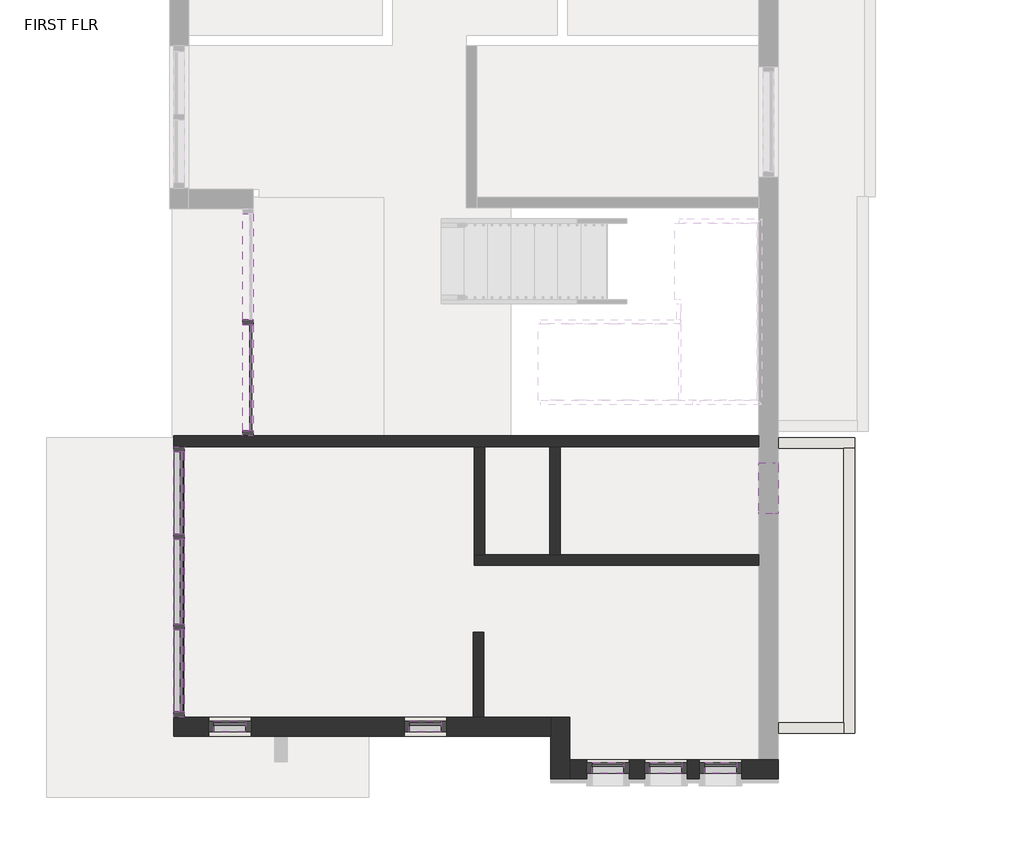
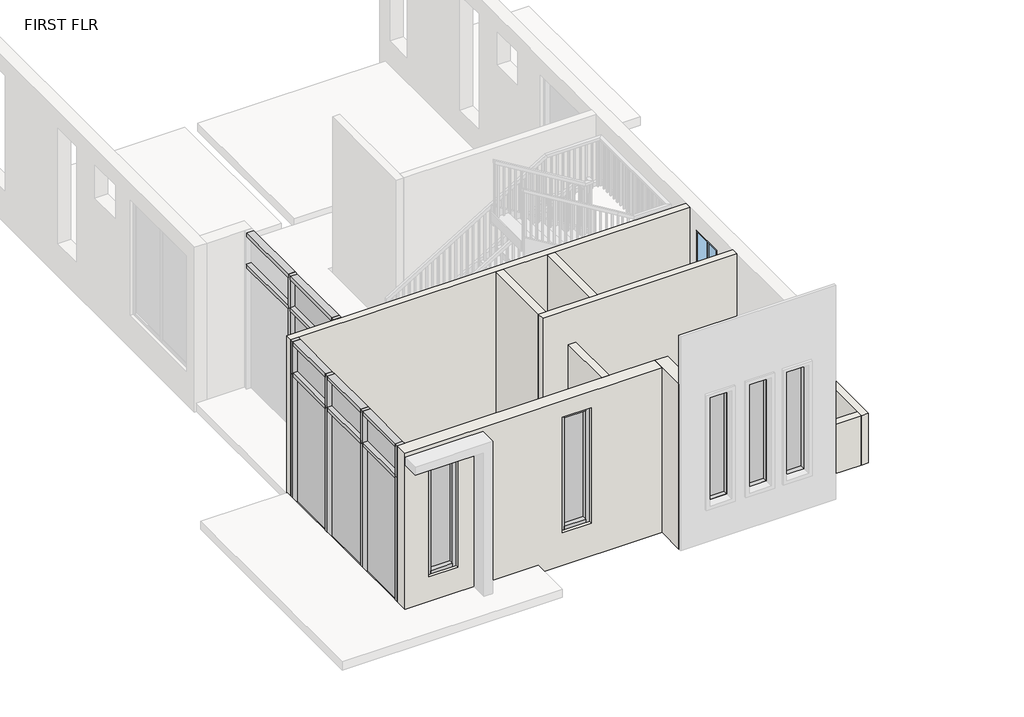
# One storey, part 1 of 4: 46 members, 13 plates, 11 walls, 1 window.
"""IFC4 building model written with IfcOpenShell, lengths in millimetres."""

from ifc_helpers import new_model, si_unit, frame, origin, place, context, project, spatial, polyline, outline, extrude, faceted_brep, transform, mapped, element, save
from components import member_f0fea5a5, member_ee409385, member_2af3cda3, member_40129ecf, member_6e77e263, member_47bfaf8a, member_1093a910, member_585633ab, member_389f1ce1, member_852ada5c, member_dfe75557, member_3374d9b6, system_panel_glazed_2be43394, system_panel_glazed_82b35773, system_panel_glazed_8cf484b6, system_panel_glazed_73690fa1, system_panel_glazed_b4437c67, system_panel_glazed_c5c5478c, system_panel_glazed_dc74cd20, window_80340324

model = new_model("IFC4")

# Units and contexts
model_context = context("Model", 3, world=origin())
ifc_project = project(units=[si_unit("LENGTHUNIT", "METRE", prefix="MILLI")], contexts=[model_context])

# Site, building, storey
site = spatial("IfcSite", under=ifc_project)
building = spatial("IfcBuilding", under=site)
storey = spatial("IfcBuildingStorey", under=building, Name="FIRST FLR", Elevation=3048.0)

# Members
placement = place(None, origin())
member_shape = member_f0fea5a5(model_context)
element("IfcMember", 1, ObjectType="Rectangular Mullion : 2.5\" x 5\" rectangular", at=placement, inside=storey, context=model_context, shape_type="MappedRepresentation", body=[
    mapped(member_shape, transform((-12015.640556, -6619.6163702, 3048.0), x_axis=(0.0, -1.0, 0.0), y_axis=(-1.0, 0.0, 0.0), z_axis=(0.0, 0.0, -1.0))),
])
element("IfcMember", 2, ObjectType="Rectangular Mullion : 2.5\" x 5\" rectangular", at=placement, inside=storey, context=model_context, shape_type="MappedRepresentation", body=[
    mapped(member_shape, transform((-12844.3906521, -9183.83582, 3048.0), x_axis=(0.0, -1.0, 0.0), y_axis=(-1.0, 0.0, 0.0), z_axis=(0.0, 0.0, -1.0))),
])
element("IfcMember", 3, ObjectType="Rectangular Mullion : 2.5\" x 5\" rectangular", at=placement, inside=storey, context=model_context, shape_type="MappedRepresentation", body=[
    mapped(member_shape, transform((-12844.3906521, -10261.7405605, 3048.0), x_axis=(0.0, -1.0, 0.0), y_axis=(-1.0, 0.0, 0.0), z_axis=(0.0, 0.0, -1.0))),
])
member_2_shape = member_ee409385(model_context)
element("IfcMember", 4, ObjectType="Rectangular Mullion : 2.5\" x 5\" rectangular", at=placement, inside=storey, context=model_context, shape_type="MappedRepresentation", body=[
    mapped(member_2_shape, transform((-12015.640556, -7978.9310793, 3048.0), x_axis=(0.0, -1.0, 0.0), y_axis=(-1.0, 0.0, 0.0), z_axis=(0.0, 0.0, -1.0))),
])
element("IfcMember", 5, ObjectType="Rectangular Mullion : 2.5\" x 5\" rectangular", at=placement, inside=storey, context=model_context, shape_type="MappedRepresentation", body=[
    mapped(member_2_shape, transform((-12844.3906521, -11339.6453012, 3048.0), x_axis=(0.0, -1.0, 0.0), y_axis=(-1.0, 0.0, 0.0), z_axis=(0.0, 0.0, -1.0))),
])
element("IfcMember", 6, ObjectType="Rectangular Mullion : 2.5\" x 5\" rectangular", at=placement, inside=storey, context=model_context, shape_type="MappedRepresentation", body=[
    mapped(member_2_shape, transform((-12844.3906521, -8105.9310793, 5486.4), x_axis=(0.0, 1.0, 0.0), y_axis=(-1.0, 0.0, 0.0), z_axis=(0.0, 0.0, 1.0))),
])
member_3_shape = member_2af3cda3(model_context)
element("IfcMember", 7, ObjectType="Rectangular Mullion : 2.5\" x 5\" rectangular", at=placement, inside=storey, context=model_context, shape_type="MappedRepresentation", body=[
    mapped(member_3_shape, transform((-12015.640556, -7915.4310793, 6096.0), x_axis=(0.0, 0.0, 1.0), y_axis=(-1.0, 0.0, 0.0), z_axis=(0.0, -1.0, 0.0))),
])
element("IfcMember", 8, ObjectType="Rectangular Mullion : 2.5\" x 5\" rectangular", at=placement, inside=storey, context=model_context, shape_type="MappedRepresentation", body=[
    mapped(member_3_shape, transform((-12015.640556, -6587.8663702, 6096.0), x_axis=(0.0, 0.0, 1.0), y_axis=(-1.0, 0.0, 0.0), z_axis=(0.0, -1.0, 0.0))),
])
element("IfcMember", 9, ObjectType="Rectangular Mullion : 2.5\" x 5\" rectangular", at=placement, inside=storey, context=model_context, shape_type="MappedRepresentation", body=[
    mapped(member_3_shape, transform((-12015.640556, -6651.3663702, 3048.0), x_axis=(0.0, 0.0, -1.0), y_axis=(-1.0, 0.0, 0.0), z_axis=(0.0, 1.0, 0.0))),
])
member_4_shape = member_40129ecf(model_context)
element("IfcMember", 10, ObjectType="Rectangular Mullion : 2.5\" x 5\" rectangular", at=placement, inside=storey, context=model_context, shape_type="MappedRepresentation", body=[
    mapped(member_4_shape, transform((-12015.640556, -6587.8663702, 5486.4), x_axis=(0.0, 0.0, 1.0), y_axis=(-1.0, 0.0, 0.0), z_axis=(0.0, -1.0, 0.0))),
])
element("IfcMember", 11, ObjectType="Rectangular Mullion : 2.5\" x 5\" rectangular", at=placement, inside=storey, context=model_context, shape_type="MappedRepresentation", body=[
    mapped(member_4_shape, transform((-12015.640556, -7915.4310793, 5486.4), x_axis=(0.0, 0.0, 1.0), y_axis=(-1.0, 0.0, 0.0), z_axis=(0.0, -1.0, 0.0))),
])
member_5_shape = member_6e77e263(model_context)
element("IfcMember", 12, ObjectType="Rectangular Mullion : 2.5\" x 5\" rectangular", at=placement, inside=storey, context=model_context, shape_type="MappedRepresentation", body=[
    mapped(member_5_shape, transform((-12015.640556, -6619.6163702, 5486.4), x_axis=(0.0, -1.0, 0.0), y_axis=(-1.0, 0.0, 0.0), z_axis=(0.0, 0.0, -1.0))),
])
element("IfcMember", 13, ObjectType="Rectangular Mullion : 2.5\" x 5\" rectangular", at=placement, inside=storey, context=model_context, shape_type="MappedRepresentation", body=[
    mapped(member_5_shape, transform((-12844.3906521, -9183.83582, 5486.4), x_axis=(0.0, -1.0, 0.0), y_axis=(-1.0, 0.0, 0.0), z_axis=(0.0, 0.0, -1.0))),
])
element("IfcMember", 14, ObjectType="Rectangular Mullion : 2.5\" x 5\" rectangular", at=placement, inside=storey, context=model_context, shape_type="MappedRepresentation", body=[
    mapped(member_5_shape, transform((-12844.3906521, -10261.7405605, 5486.4), x_axis=(0.0, -1.0, 0.0), y_axis=(-1.0, 0.0, 0.0), z_axis=(0.0, 0.0, -1.0))),
])
member_6_shape = member_47bfaf8a(model_context)
element("IfcMember", 15, ObjectType="Rectangular Mullion : 2.5\" x 5\" rectangular", at=placement, inside=storey, context=model_context, shape_type="MappedRepresentation", body=[
    mapped(member_6_shape, transform((-12844.3906521, -8105.9310793, 6096.0), x_axis=(0.0, 1.0, 0.0), y_axis=(-1.0, 0.0, 0.0), z_axis=(0.0, 0.0, 1.0))),
])
element("IfcMember", 16, ObjectType="Rectangular Mullion : 2.5\" x 5\" rectangular", at=placement, inside=storey, context=model_context, shape_type="MappedRepresentation", body=[
    mapped(member_6_shape, transform((-12015.640556, -7978.9310793, 5486.4), x_axis=(0.0, -1.0, 0.0), y_axis=(-1.0, 0.0, 0.0), z_axis=(0.0, 0.0, -1.0))),
])
element("IfcMember", 17, ObjectType="Rectangular Mullion : 2.5\" x 5\" rectangular", at=placement, inside=storey, context=model_context, shape_type="MappedRepresentation", body=[
    mapped(member_6_shape, transform((-12844.3906521, -11339.6453012, 5486.4), x_axis=(0.0, -1.0, 0.0), y_axis=(-1.0, 0.0, 0.0), z_axis=(0.0, 0.0, -1.0))),
])
member_7_shape = member_1093a910(model_context)
element("IfcMember", 18, ObjectType="Rectangular Mullion : 2.5\" x 5\" rectangular", at=placement, inside=storey, context=model_context, shape_type="MappedRepresentation", body=[
    mapped(member_7_shape, transform((-12844.3906521, -11276.1453012, 6096.0), x_axis=(0.0, 0.0, 1.0), y_axis=(-1.0, 0.0, 0.0), z_axis=(0.0, -1.0, 0.0))),
])
element("IfcMember", 19, ObjectType="Rectangular Mullion : 2.5\" x 5\" rectangular", at=placement, inside=storey, context=model_context, shape_type="MappedRepresentation", body=[
    mapped(member_7_shape, transform((-12844.3906521, -9152.08582, 6096.0), x_axis=(0.0, 0.0, 1.0), y_axis=(-1.0, 0.0, 0.0), z_axis=(0.0, -1.0, 0.0))),
])
element("IfcMember", 20, ObjectType="Rectangular Mullion : 2.5\" x 5\" rectangular", at=placement, inside=storey, context=model_context, shape_type="MappedRepresentation", body=[
    mapped(member_7_shape, transform((-12844.3906521, -8169.4310793, 3048.0), x_axis=(0.0, 0.0, -1.0), y_axis=(-1.0, 0.0, 0.0), z_axis=(0.0, 1.0, 0.0))),
])
element("IfcMember", 21, ObjectType="Rectangular Mullion : 2.5\" x 5\" rectangular", at=placement, inside=storey, context=model_context, shape_type="MappedRepresentation", body=[
    mapped(member_7_shape, transform((-12844.3906521, -10293.4905605, 3048.0), x_axis=(0.0, 0.0, -1.0), y_axis=(-1.0, 0.0, 0.0), z_axis=(0.0, 1.0, 0.0))),
])
member_8_shape = member_585633ab(model_context)
element("IfcMember", 22, ObjectType="Rectangular Mullion : 2.5\" x 5\" rectangular", at=placement, inside=storey, context=model_context, shape_type="MappedRepresentation", body=[
    mapped(member_8_shape, transform((-12844.3906521, -10229.9905605, 6096.0), x_axis=(0.0, 0.0, 1.0), y_axis=(-1.0, 0.0, 0.0), z_axis=(0.0, -1.0, 0.0))),
])
element("IfcMember", 23, ObjectType="Rectangular Mullion : 2.5\" x 5\" rectangular", at=placement, inside=storey, context=model_context, shape_type="MappedRepresentation", body=[
    mapped(member_8_shape, transform((-12844.3906521, -9215.58582, 3048.0), x_axis=(0.0, 0.0, -1.0), y_axis=(-1.0, 0.0, 0.0), z_axis=(0.0, 1.0, 0.0))),
])
member_9_shape = member_389f1ce1(model_context)
element("IfcMember", 24, ObjectType="Rectangular Mullion : 2.5\" x 5\" rectangular", at=placement, inside=storey, context=model_context, shape_type="MappedRepresentation", body=[
    mapped(member_9_shape, transform((-12844.3906521, -9152.08582, 5486.4), x_axis=(0.0, 0.0, 1.0), y_axis=(-1.0, 0.0, 0.0), z_axis=(0.0, -1.0, 0.0))),
])
element("IfcMember", 25, ObjectType="Rectangular Mullion : 2.5\" x 5\" rectangular", at=placement, inside=storey, context=model_context, shape_type="MappedRepresentation", body=[
    mapped(member_9_shape, transform((-12844.3906521, -11276.1453012, 5486.4), x_axis=(0.0, 0.0, 1.0), y_axis=(-1.0, 0.0, 0.0), z_axis=(0.0, -1.0, 0.0))),
])
member_10_shape = member_852ada5c(model_context)
element("IfcMember", 26, ObjectType="Rectangular Mullion : 2.5\" x 5\" rectangular", at=placement, inside=storey, context=model_context, shape_type="MappedRepresentation", body=[
    mapped(member_10_shape, transform((-12844.3906521, -10229.9905605, 5486.4), x_axis=(0.0, 0.0, 1.0), y_axis=(-1.0, 0.0, 0.0), z_axis=(0.0, -1.0, 0.0))),
])
member_11_shape = member_dfe75557(model_context)
element("IfcMember", 27, ObjectType="Rectangular Mullion : 2.5\" x 5\" rectangular", at=placement, inside=storey, context=model_context, shape_type="MappedRepresentation", body=[
    mapped(member_11_shape, transform((-7523.7171142, -11945.8509606, 5791.2), x_axis=(0.0, 0.0, 1.0), y_axis=(0.0, -1.0, 0.0), z_axis=(1.0, 0.0, 0.0))),
])
element("IfcMember", 28, ObjectType="Rectangular Mullion : 2.5\" x 5\" rectangular", at=placement, inside=storey, context=model_context, shape_type="MappedRepresentation", body=[
    mapped(member_11_shape, transform((-6831.5671142, -11945.8509606, 5791.2), x_axis=(0.0, 0.0, 1.0), y_axis=(0.0, -1.0, 0.0), z_axis=(1.0, 0.0, 0.0))),
])
element("IfcMember", 29, ObjectType="Rectangular Mullion : 2.5\" x 5\" rectangular", at=placement, inside=storey, context=model_context, shape_type="MappedRepresentation", body=[
    mapped(member_11_shape, transform((-6177.5171142, -11945.8509606, 5791.2), x_axis=(0.0, 0.0, 1.0), y_axis=(0.0, -1.0, 0.0), z_axis=(1.0, 0.0, 0.0))),
])
element("IfcMember", 30, ObjectType="Rectangular Mullion : 2.5\" x 5\" rectangular", at=placement, inside=storey, context=model_context, shape_type="MappedRepresentation", body=[
    mapped(member_11_shape, transform((-9707.4906521, -11453.9453012, 5791.2), x_axis=(0.0, 0.0, 1.0), y_axis=(0.0, -1.0, 0.0), z_axis=(1.0, 0.0, 0.0))),
])
element("IfcMember", 31, ObjectType="Rectangular Mullion : 2.5\" x 5\" rectangular", at=placement, inside=storey, context=model_context, shape_type="MappedRepresentation", body=[
    mapped(member_11_shape, transform((-12044.2906521, -11453.9453012, 5791.2), x_axis=(0.0, 0.0, 1.0), y_axis=(0.0, -1.0, 0.0), z_axis=(1.0, 0.0, 0.0))),
])
element("IfcMember", 32, ObjectType="Rectangular Mullion : 2.5\" x 5\" rectangular", at=placement, inside=storey, context=model_context, shape_type="MappedRepresentation", body=[
    mapped(member_11_shape, transform((-7904.7171142, -11945.8509606, 3657.6), x_axis=(0.0, 0.0, -1.0), y_axis=(0.0, -1.0, 0.0), z_axis=(-1.0, 0.0, 0.0))),
])
element("IfcMember", 33, ObjectType="Rectangular Mullion : 2.5\" x 5\" rectangular", at=placement, inside=storey, context=model_context, shape_type="MappedRepresentation", body=[
    mapped(member_11_shape, transform((-7212.5671142, -11945.8509606, 3657.6), x_axis=(0.0, 0.0, -1.0), y_axis=(0.0, -1.0, 0.0), z_axis=(-1.0, 0.0, 0.0))),
])
element("IfcMember", 34, ObjectType="Rectangular Mullion : 2.5\" x 5\" rectangular", at=placement, inside=storey, context=model_context, shape_type="MappedRepresentation", body=[
    mapped(member_11_shape, transform((-6558.5171142, -11945.8509606, 3657.6), x_axis=(0.0, 0.0, -1.0), y_axis=(0.0, -1.0, 0.0), z_axis=(-1.0, 0.0, 0.0))),
])
element("IfcMember", 35, ObjectType="Rectangular Mullion : 2.5\" x 5\" rectangular", at=placement, inside=storey, context=model_context, shape_type="MappedRepresentation", body=[
    mapped(member_11_shape, transform((-10088.4906521, -11453.9453012, 3657.6), x_axis=(0.0, 0.0, -1.0), y_axis=(0.0, -1.0, 0.0), z_axis=(-1.0, 0.0, 0.0))),
])
element("IfcMember", 36, ObjectType="Rectangular Mullion : 2.5\" x 5\" rectangular", at=placement, inside=storey, context=model_context, shape_type="MappedRepresentation", body=[
    mapped(member_11_shape, transform((-12425.2906521, -11453.9453012, 3657.6), x_axis=(0.0, 0.0, -1.0), y_axis=(0.0, -1.0, 0.0), z_axis=(-1.0, 0.0, 0.0))),
])
member_12_shape = member_3374d9b6(model_context)
element("IfcMember", 37, ObjectType="Rectangular Mullion : 2.5\" x 5\" rectangular", at=placement, inside=storey, context=model_context, shape_type="MappedRepresentation", body=[
    mapped(member_12_shape, transform((-7460.2171142, -11945.8509606, 3657.6), x_axis=(1.0, 0.0, 0.0), y_axis=(0.0, -1.0, 0.0), z_axis=(0.0, 0.0, -1.0))),
])
element("IfcMember", 38, ObjectType="Rectangular Mullion : 2.5\" x 5\" rectangular", at=placement, inside=storey, context=model_context, shape_type="MappedRepresentation", body=[
    mapped(member_12_shape, transform((-6768.0671142, -11945.8509606, 3657.6), x_axis=(1.0, 0.0, 0.0), y_axis=(0.0, -1.0, 0.0), z_axis=(0.0, 0.0, -1.0))),
])
element("IfcMember", 39, ObjectType="Rectangular Mullion : 2.5\" x 5\" rectangular", at=placement, inside=storey, context=model_context, shape_type="MappedRepresentation", body=[
    mapped(member_12_shape, transform((-6114.0171142, -11945.8509606, 3657.6), x_axis=(1.0, 0.0, 0.0), y_axis=(0.0, -1.0, 0.0), z_axis=(0.0, 0.0, -1.0))),
])
element("IfcMember", 40, ObjectType="Rectangular Mullion : 2.5\" x 5\" rectangular", at=placement, inside=storey, context=model_context, shape_type="MappedRepresentation", body=[
    mapped(member_12_shape, transform((-9643.9906521, -11453.9453012, 3657.6), x_axis=(1.0, 0.0, 0.0), y_axis=(0.0, -1.0, 0.0), z_axis=(0.0, 0.0, -1.0))),
])
element("IfcMember", 41, ObjectType="Rectangular Mullion : 2.5\" x 5\" rectangular", at=placement, inside=storey, context=model_context, shape_type="MappedRepresentation", body=[
    mapped(member_12_shape, transform((-11980.7906521, -11453.9453012, 3657.6), x_axis=(1.0, 0.0, 0.0), y_axis=(0.0, -1.0, 0.0), z_axis=(0.0, 0.0, -1.0))),
])
element("IfcMember", 42, ObjectType="Rectangular Mullion : 2.5\" x 5\" rectangular", at=placement, inside=storey, context=model_context, shape_type="MappedRepresentation", body=[
    mapped(member_12_shape, transform((-7968.2171142, -11945.8509606, 5791.2), x_axis=(-1.0, 0.0, 0.0), y_axis=(0.0, -1.0, 0.0), z_axis=(0.0, 0.0, 1.0))),
])
element("IfcMember", 43, ObjectType="Rectangular Mullion : 2.5\" x 5\" rectangular", at=placement, inside=storey, context=model_context, shape_type="MappedRepresentation", body=[
    mapped(member_12_shape, transform((-7276.0671142, -11945.8509606, 5791.2), x_axis=(-1.0, 0.0, 0.0), y_axis=(0.0, -1.0, 0.0), z_axis=(0.0, 0.0, 1.0))),
])
element("IfcMember", 44, ObjectType="Rectangular Mullion : 2.5\" x 5\" rectangular", at=placement, inside=storey, context=model_context, shape_type="MappedRepresentation", body=[
    mapped(member_12_shape, transform((-6622.0171142, -11945.8509606, 5791.2), x_axis=(-1.0, 0.0, 0.0), y_axis=(0.0, -1.0, 0.0), z_axis=(0.0, 0.0, 1.0))),
])
element("IfcMember", 45, ObjectType="Rectangular Mullion : 2.5\" x 5\" rectangular", at=placement, inside=storey, context=model_context, shape_type="MappedRepresentation", body=[
    mapped(member_12_shape, transform((-10151.9906521, -11453.9453012, 5791.2), x_axis=(-1.0, 0.0, 0.0), y_axis=(0.0, -1.0, 0.0), z_axis=(0.0, 0.0, 1.0))),
])
element("IfcMember", 46, ObjectType="Rectangular Mullion : 2.5\" x 5\" rectangular", at=placement, inside=storey, context=model_context, shape_type="MappedRepresentation", body=[
    mapped(member_12_shape, transform((-12488.7906521, -11453.9453012, 5791.2), x_axis=(-1.0, 0.0, 0.0), y_axis=(0.0, -1.0, 0.0), z_axis=(0.0, 0.0, 1.0))),
])

# Plates
system_panel_glazed_shape = system_panel_glazed_2be43394(model_context)
element("IfcPlate", 47, ObjectType="System Panel : Glazed", at=placement, inside=storey, context=model_context, shape_type="MappedRepresentation", body=[
    mapped(system_panel_glazed_shape, transform((-12015.640556, -7283.3987247, 3111.5), x_axis=(0.0, -1.0, 0.0), y_axis=(1.0, 0.0, 0.0), z_axis=(0.0, 0.0, 1.0))),
])
system_panel_glazed_2_shape = system_panel_glazed_82b35773(model_context)
element("IfcPlate", 48, ObjectType="System Panel : Glazed", at=placement, inside=storey, context=model_context, shape_type="MappedRepresentation", body=[
    mapped(system_panel_glazed_2_shape, transform((-12015.640556, -7283.3987247, 5518.15), x_axis=(0.0, -1.0, 0.0), y_axis=(1.0, 0.0, 0.0), z_axis=(0.0, 0.0, 1.0))),
])
system_panel_glazed_3_shape = system_panel_glazed_8cf484b6(model_context)
element("IfcPlate", 49, ObjectType="System Panel : Glazed", at=placement, inside=storey, context=model_context, shape_type="MappedRepresentation", body=[
    mapped(system_panel_glazed_3_shape, transform((-12844.3906521, -8660.7584496, 3111.5), x_axis=(0.0, -1.0, 0.0), y_axis=(1.0, 0.0, 0.0), z_axis=(0.0, 0.0, 1.0))),
])
element("IfcPlate", 50, ObjectType="System Panel : Glazed", at=placement, inside=storey, context=model_context, shape_type="MappedRepresentation", body=[
    mapped(system_panel_glazed_3_shape, transform((-12844.3906521, -10784.8179308, 3111.5), x_axis=(0.0, -1.0, 0.0), y_axis=(1.0, 0.0, 0.0), z_axis=(0.0, 0.0, 1.0))),
])
system_panel_glazed_4_shape = system_panel_glazed_73690fa1(model_context)
element("IfcPlate", 51, ObjectType="System Panel : Glazed", at=placement, inside=storey, context=model_context, shape_type="MappedRepresentation", body=[
    mapped(system_panel_glazed_4_shape, transform((-12844.3906521, -9722.7881902, 3111.5), x_axis=(0.0, -1.0, 0.0), y_axis=(1.0, 0.0, 0.0), z_axis=(0.0, 0.0, 1.0))),
])
system_panel_glazed_5_shape = system_panel_glazed_b4437c67(model_context)
element("IfcPlate", 52, ObjectType="System Panel : Glazed", at=placement, inside=storey, context=model_context, shape_type="MappedRepresentation", body=[
    mapped(system_panel_glazed_5_shape, transform((-12844.3906521, -8660.7584496, 5518.15), x_axis=(0.0, -1.0, 0.0), y_axis=(1.0, 0.0, 0.0), z_axis=(0.0, 0.0, 1.0))),
])
element("IfcPlate", 53, ObjectType="System Panel : Glazed", at=placement, inside=storey, context=model_context, shape_type="MappedRepresentation", body=[
    mapped(system_panel_glazed_5_shape, transform((-12844.3906521, -10784.8179308, 5518.15), x_axis=(0.0, -1.0, 0.0), y_axis=(1.0, 0.0, 0.0), z_axis=(0.0, 0.0, 1.0))),
])
system_panel_glazed_6_shape = system_panel_glazed_c5c5478c(model_context)
element("IfcPlate", 54, ObjectType="System Panel : Glazed", at=placement, inside=storey, context=model_context, shape_type="MappedRepresentation", body=[
    mapped(system_panel_glazed_6_shape, transform((-12844.3906521, -9722.7881902, 5518.15), x_axis=(0.0, -1.0, 0.0), y_axis=(1.0, 0.0, 0.0), z_axis=(0.0, 0.0, 1.0))),
])
system_panel_glazed_7_shape = system_panel_glazed_dc74cd20(model_context)
element("IfcPlate", 55, ObjectType="System Panel : Glazed", at=placement, inside=storey, context=model_context, shape_type="MappedRepresentation", body=[
    mapped(system_panel_glazed_7_shape, transform((-7714.2171142, -11945.8509606, 3721.1), x_axis=(1.0, 0.0, 0.0), y_axis=(0.0, 1.0, 0.0), z_axis=(0.0, 0.0, 1.0))),
])
element("IfcPlate", 56, ObjectType="System Panel : Glazed", at=placement, inside=storey, context=model_context, shape_type="MappedRepresentation", body=[
    mapped(system_panel_glazed_7_shape, transform((-7022.0671142, -11945.8509606, 3721.1), x_axis=(1.0, 0.0, 0.0), y_axis=(0.0, 1.0, 0.0), z_axis=(0.0, 0.0, 1.0))),
])
element("IfcPlate", 57, ObjectType="System Panel : Glazed", at=placement, inside=storey, context=model_context, shape_type="MappedRepresentation", body=[
    mapped(system_panel_glazed_7_shape, transform((-6368.0171142, -11945.8509606, 3721.1), x_axis=(1.0, 0.0, 0.0), y_axis=(0.0, 1.0, 0.0), z_axis=(0.0, 0.0, 1.0))),
])
element("IfcPlate", 58, ObjectType="System Panel : Glazed", at=placement, inside=storey, context=model_context, shape_type="MappedRepresentation", body=[
    mapped(system_panel_glazed_7_shape, transform((-9897.9906521, -11453.9453012, 3721.1), x_axis=(1.0, 0.0, 0.0), y_axis=(0.0, 1.0, 0.0), z_axis=(0.0, 0.0, 1.0))),
])
element("IfcPlate", 59, ObjectType="System Panel : Glazed", at=placement, inside=storey, context=model_context, shape_type="MappedRepresentation", body=[
    mapped(system_panel_glazed_7_shape, transform((-12234.7906521, -11453.9453012, 3721.1), x_axis=(1.0, 0.0, 0.0), y_axis=(0.0, 1.0, 0.0), z_axis=(0.0, 0.0, 1.0))),
])

# Walls
element("IfcWall", 60, ObjectType="EXTERIOR WALL 9\"", at=placement, inside=storey, context=model_context, shape_type="Brep", body=[
    faceted_brep([(-12907.8906521, -11568.2453012, 3048.0), (-8399.3906521, -11568.2453012, 3048.0), (-8399.3906521, -11568.2453012, 6096.0), (-12907.8906521, -11568.2453012, 6096.0), (-10151.9906521, -11568.2453012, 3657.6), (-10151.9906521, -11568.2453012, 5791.2), (-9643.9906521, -11568.2453012, 5791.2), (-9643.9906521, -11568.2453012, 3657.6), (-12488.7906521, -11568.2453012, 3657.6), (-12488.7906521, -11568.2453012, 5791.2), (-11980.7906521, -11568.2453012, 5791.2), (-11980.7906521, -11568.2453012, 3657.6), (-8399.3906521, -11339.6453012, 3048.0), (-9199.4906521, -11339.6453012, 3048.0), (-9326.4906521, -11339.6453012, 3048.0), (-12907.8906521, -11339.6453012, 3048.0), (-12907.8906521, -11339.6453012, 6096.0), (-9326.4906521, -11339.6453012, 6096.0), (-9199.4906521, -11339.6453012, 6096.0), (-8399.3906521, -11339.6453012, 6096.0), (-10151.9906521, -11339.6453012, 5791.2), (-10151.9906521, -11339.6453012, 3657.6), (-9643.9906521, -11339.6453012, 3657.6), (-9643.9906521, -11339.6453012, 5791.2), (-12488.7906521, -11339.6453012, 5791.2), (-12488.7906521, -11339.6453012, 3657.6), (-11980.7906521, -11339.6453012, 3657.6), (-11980.7906521, -11339.6453012, 5791.2)], [[[0, 1, 2, 3], [4, 5, 6, 7], [8, 9, 10, 11]], [[12, 13, 14, 15, 16, 17, 18, 19], [20, 21, 22, 23], [24, 25, 26, 27]], [[1, 0, 15, 14, 13, 12]], [[3, 2, 19, 18, 17, 16]], [[0, 3, 16, 15]], [[2, 1, 12, 19]], [[4, 21, 20, 5]], [[5, 20, 23, 6]], [[6, 23, 22, 7]], [[21, 4, 7, 22]], [[24, 9, 8, 25]], [[9, 24, 27, 10]], [[10, 27, 26, 11]], [[25, 8, 11, 26]]]),
])
element("IfcWall", 61, ObjectType="EXTERIOR WALL 9\"", at=placement, inside=storey, context=model_context, shape_type="Brep", body=[
    faceted_brep([(-8399.3906521, -11339.6453012, 3048.0), (-8399.3906521, -11568.2453012, 3048.0), (-8399.3906521, -12076.2453012, 3048.0), (-8399.3906521, -12076.2453012, 6096.0), (-8399.3906521, -11568.2453012, 6096.0), (-8399.3906521, -11339.6453012, 6096.0), (-8170.7906521, -11339.6453012, 3048.0), (-8170.7906521, -11339.6453012, 6096.0), (-8170.7906521, -11847.6453012, 6096.0), (-8170.7906521, -12076.2453012, 6096.0), (-8170.7906521, -12076.2453012, 3048.0), (-8170.7906521, -11847.6453012, 3048.0)], [[[0, 1, 2, 3, 4, 5]], [[6, 7, 8, 9, 10, 11]], [[2, 1, 0, 6, 11, 10]], [[5, 4, 3, 9, 8, 7]], [[0, 5, 7, 6]], [[3, 2, 10, 9]]]),
])
element("IfcWall", 62, ObjectType="EXTERIOR WALL 9\"", at=placement, inside=storey, context=model_context, shape_type="Brep", body=[
    faceted_brep([(-8170.7906521, -12076.2453012, 3048.0), (-5681.5906521, -12076.2453012, 3048.0), (-5681.5906521, -12076.2453012, 6096.0), (-8170.7906521, -12076.2453012, 6096.0), (-7968.2171142, -12076.2453012, 3657.6), (-7968.2171142, -12076.2453012, 5791.2), (-7460.2171142, -12076.2453012, 5791.2), (-7460.2171142, -12076.2453012, 3657.6), (-7276.0671142, -12076.2453012, 3657.6), (-7276.0671142, -12076.2453012, 5791.2), (-6768.0671142, -12076.2453012, 5791.2), (-6768.0671142, -12076.2453012, 3657.6), (-6622.0171142, -12076.2453012, 3657.6), (-6622.0171142, -12076.2453012, 5791.2), (-6114.0171142, -12076.2453012, 5791.2), (-6114.0171142, -12076.2453012, 3657.6), (-5681.5906521, -11847.6453012, 3048.0), (-5910.1906521, -11847.6453012, 3048.0), (-8170.7906521, -11847.6453012, 3048.0), (-8170.7906521, -11847.6453012, 6096.0), (-5910.1906521, -11847.6453012, 6096.0), (-5681.5906521, -11847.6453012, 6096.0), (-7968.2171142, -11847.6453012, 5791.2), (-7968.2171142, -11847.6453012, 3657.6), (-7460.2171142, -11847.6453012, 3657.6), (-7460.2171142, -11847.6453012, 5791.2), (-7276.0671142, -11847.6453012, 5791.2), (-7276.0671142, -11847.6453012, 3657.6), (-6768.0671142, -11847.6453012, 3657.6), (-6768.0671142, -11847.6453012, 5791.2), (-6622.0171142, -11847.6453012, 5791.2), (-6622.0171142, -11847.6453012, 3657.6), (-6114.0171142, -11847.6453012, 3657.6), (-6114.0171142, -11847.6453012, 5791.2)], [[[0, 1, 2, 3], [4, 5, 6, 7], [8, 9, 10, 11], [12, 13, 14, 15]], [[16, 17, 18, 19, 20, 21], [22, 23, 24, 25], [26, 27, 28, 29], [30, 31, 32, 33]], [[1, 0, 18, 17, 16]], [[3, 2, 21, 20, 19]], [[0, 3, 19, 18]], [[2, 1, 16, 21]], [[4, 23, 22, 5]], [[5, 22, 25, 6]], [[6, 25, 24, 7]], [[23, 4, 7, 24]], [[8, 27, 26, 9]], [[9, 26, 29, 10]], [[28, 11, 10, 29]], [[27, 8, 11, 28]], [[12, 31, 30, 13]], [[13, 30, 33, 14]], [[32, 15, 14, 33]], [[31, 12, 15, 32]]]),
])
element("IfcWall", 63, ObjectType="INTERIOR WALL PAINT 5\"", at=placement, inside=storey, context=model_context, shape_type="Brep", body=[
    faceted_brep([(-5910.1906521, -7978.9310793, 3048.0), (-12907.8906521, -7978.9310793, 3048.0), (-12907.8906521, -7978.9310793, 6096.0), (-5910.1906521, -7978.9310793, 6096.0), (-5910.1906521, -8105.9310793, 3048.0), (-5910.1906521, -8105.9310793, 6096.0), (-8285.0906521, -8105.9310793, 6096.0), (-8412.0906521, -8105.9310793, 6096.0), (-9186.7906521, -8105.9310793, 6096.0), (-9313.7906521, -8105.9310793, 6096.0), (-12907.8906521, -8105.9310793, 6096.0), (-12907.8906521, -8105.9310793, 3048.0), (-9313.7906521, -8105.9310793, 3048.0), (-9186.7906521, -8105.9310793, 3048.0), (-8412.0906521, -8105.9310793, 3048.0), (-8285.0906521, -8105.9310793, 3048.0)], [[[0, 1, 2, 3]], [[4, 5, 6, 7, 8, 9, 10, 11, 12, 13, 14, 15]], [[1, 0, 4, 15, 14, 13, 12, 11]], [[2, 1, 11, 10]], [[3, 2, 10, 9, 8, 7, 6, 5]], [[0, 3, 5, 4]]]),
])
element("IfcWall", 64, ObjectType="INTERIOR WALL PAINT 5\"", at=placement, inside=storey, context=model_context, shape_type="Brep", body=[
    faceted_brep([(-5910.1906521, -9397.5830995, 3048.0), (-8285.0906521, -9397.5830995, 3048.0), (-8412.0906521, -9397.5830995, 3048.0), (-9186.7906521, -9397.5830995, 3048.0), (-9313.7906521, -9397.5830995, 3048.0), (-9313.7906521, -9397.5830995, 6096.0), (-9186.7906521, -9397.5830995, 6096.0), (-8412.0906521, -9397.5830995, 6096.0), (-8285.0906521, -9397.5830995, 6096.0), (-5910.1906521, -9397.5830995, 6096.0), (-5910.1906521, -9524.5830995, 3048.0), (-5910.1906521, -9524.5830995, 6096.0), (-9313.7906521, -9524.5830995, 6096.0), (-9313.7906521, -9524.5830995, 3048.0)], [[[0, 1, 2, 3, 4, 5, 6, 7, 8, 9]], [[10, 11, 12, 13]], [[4, 3, 2, 1, 0, 10, 13]], [[9, 8, 7, 6, 5, 12, 11]], [[0, 9, 11, 10]], [[5, 4, 13, 12]]]),
])
element("IfcWall", 65, ObjectType="INTERIOR WALL PAINT 5\"", at=placement, inside=storey, context=model_context, shape_type="SweptSolid", body=[
    extrude(outline(polyline([(-9186.7906521, -8105.9310793), (-9186.7906521, -9397.5830995), (-9313.7906521, -9397.5830995), (-9313.7906521, -8105.9310793), (-9186.7906521, -8105.9310793)])), frame((0.0, 0.0, 3048.0), z_axis=(0.0, 0.0, 1.0), x_axis=(1.0, 0.0, 0.0)), (0.0, 0.0, 1.0), 3048.0),
])
element("IfcWall", 66, ObjectType="INTERIOR WALL PAINT 5\"", at=placement, inside=storey, context=model_context, shape_type="SweptSolid", body=[
    extrude(outline(polyline([(-8412.0906521, -9397.5830995), (-8412.0906521, -8105.9310793), (-8285.0906521, -8105.9310793), (-8285.0906521, -9397.5830995), (-8412.0906521, -9397.5830995)])), frame((0.0, 0.0, 3048.0), z_axis=(0.0, 0.0, 1.0), x_axis=(1.0, 0.0, 0.0)), (0.0, 0.0, 1.0), 3048.0),
])
element("IfcWall", 67, ObjectType="INTERIOR WALL PAINT 5\"", at=placement, inside=storey, context=model_context, shape_type="SweptSolid", body=[
    extrude(outline(polyline([(-9199.4906521, -10323.6453012), (-9199.4906521, -11339.6453012), (-9326.4906521, -11339.6453012), (-9326.4906521, -10323.6453012), (-9199.4906521, -10323.6453012)])), frame((0.0, 0.0, 3048.0), z_axis=(0.0, 0.0, 1.0), x_axis=(1.0, 0.0, 0.0)), (0.0, 0.0, 1.0), 3048.0),
])
element("IfcWall", 68, ObjectType="INTERIOR WALL PAINT 5\"", at=placement, inside=storey, context=model_context, shape_type="Brep", body=[
    faceted_brep([(-5681.5906521, -8124.9810793, 3048.0), (-4894.1906521, -8124.9810793, 3048.0), (-4767.1906521, -8124.9810793, 3048.0), (-4767.1906521, -8124.9810793, 3962.4), (-4894.1906521, -8124.9810793, 3962.4), (-5681.5906521, -8124.9810793, 3962.4), (-5681.5906521, -7997.9810793, 3048.0), (-5681.5906521, -7997.9810793, 3962.4), (-4767.1906521, -7997.9810793, 3962.4), (-4767.1906521, -7997.9810793, 3048.0)], [[[0, 1, 2, 3, 4, 5]], [[6, 7, 8, 9]], [[2, 1, 0, 6, 9]], [[5, 4, 3, 8, 7]], [[0, 5, 7, 6]], [[3, 2, 9, 8]]]),
])
element("IfcWall", 69, ObjectType="INTERIOR WALL PAINT 5\"", at=placement, inside=storey, context=model_context, shape_type="Brep", body=[
    faceted_brep([(-4894.1906521, -8124.9810793, 3048.0), (-4894.1906521, -11407.9310793, 3048.0), (-4894.1906521, -11534.9310793, 3048.0), (-4894.1906521, -11534.9310793, 3962.4), (-4894.1906521, -11407.9310793, 3962.4), (-4894.1906521, -8124.9810793, 3962.4), (-4767.1906521, -8124.9810793, 3048.0), (-4767.1906521, -8124.9810793, 3962.4), (-4767.1906521, -11534.9310793, 3962.4), (-4767.1906521, -11534.9310793, 3048.0)], [[[0, 1, 2, 3, 4, 5]], [[6, 7, 8, 9]], [[2, 1, 0, 6, 9]], [[5, 4, 3, 8, 7]], [[0, 5, 7, 6]], [[3, 2, 9, 8]]]),
])
element("IfcWall", 70, ObjectType="INTERIOR WALL PAINT 5\"", at=placement, inside=storey, context=model_context, shape_type="SweptSolid", body=[
    extrude(outline(polyline([(-5681.5906521, -11407.9310793), (-4894.1906521, -11407.9310793), (-4894.1906521, -11534.9310793), (-5681.5906521, -11534.9310793), (-5681.5906521, -11407.9310793)])), frame((0.0, 0.0, 3048.0), z_axis=(0.0, 0.0, 1.0), x_axis=(1.0, 0.0, 0.0)), (0.0, 0.0, 1.0), 914.4),
])

# Window
window_shape = window_80340324(model_context)
element("IfcWindow", 71, ObjectType="Fixed : 24\" x 24\"", at=placement, inside=storey, context=model_context, shape_type="MappedRepresentation", body=[
    mapped(window_shape, transform((-5795.8906521, -8639.3310793, 4267.2), x_axis=(0.0, -1.0, 0.0), y_axis=(1.0, 0.0, 0.0), z_axis=(0.0, 0.0, 1.0))),
])

save(model, "model.ifc")

# Revit data of these elements
# Type "Rectangular Mullion : 2.5\" x 5\" rectangular"
#   built-in parameter 1007304 = 0.416667 (stored number, unit not read)
#   built-in parameter 1007301 = 0.104167 (stored number, unit not read)
#   built-in parameter 1007300 = 0.104167 (stored number, unit not read)
# Type "System Panel : Glazed"
#   Construction Type Id = "GSP4R"
#   Analytic Construction = "1/8 in Pilkington single glazing"
#   Visual Light Transmittance = 0.9
#   Solar Heat Gain Coefficient = 0.86
#   Heat Transfer Coefficient (U) = 1.18115 BTU/(h·ft²·°F)
#   Define Thermal Properties by = 1
# Type "EXTERIOR WALL 9\""
#   Assembly Code = "B2010"
#   Layers, outside or top first: 0' - 9" "EXTERIOR WALL PAINT" (function 1)
# Type "INTERIOR WALL PAINT 5\""
#   Assembly Code = "B2010"
#   Layers, outside or top first: 0' - 5" "EXTERIOR WALL PAINT" (function 1)
# Type "Fixed : 24\" x 24\""
#   Type Mark = "3"
#   Construction Type Id = "GSP4R"
#   Assembly Code = "B2020100"
#   Analytic Construction = "1/8 in Pilkington single glazing"
#   Visual Light Transmittance = 0.9
#   Solar Heat Gain Coefficient = 0.78
#   Heat Transfer Coefficient (U) = 0.6496 BTU/(h·ft²·°F)
#   Height = 2' - 0"
#   Default Sill Height = 3' - 0"
#   Width = 2' - 0"
#   Window Inset = 0' - 0 3/4"
#   Define Thermal Properties by = 1
#   Define Thermal Properties by = 1
#   Glass Pane Material = Glass
#   Sash Material = Sash
#   Wall Closure = (empty or 0)
# Elements 1, 2, 3, 4, 5, 6, 7, 8, 9, 10, 11, 12, 13, 14, 15, 16, 17, 18, 19, 20, 21, 22, 23, 24, 25, 26, 27, 28, 29, 30, 31, 32, 33, 34, 35, 36, 37, 38, 39, 40, 41, 42, 43, 44, 45, 46 (IfcMember, "Rectangular Mullion : 2.5\" x 5\" rectangular")
#   Phase Created = New Construction
# Elements 47, 48, 49, 50, 51, 52, 53, 54, 55, 56, 57, 58, 59 (IfcPlate, "System Panel : Glazed")
#   Phase Created = New Construction
#   Materials on its faces: "Glass"
# Elements 60, 61, 62 (IfcWall, "EXTERIOR WALL 9\"")
#   Top Offset = 0' - 0"
#   Base Offset = 0' - 0"
#   wall height = 10' - 0"
#   Phase Created = New Construction
#   Base Constraint = FIRST FLR
#   Top Constraint = SECOND FLR
#   Materials on its faces: "EXTERIOR WALL PAINT"
# Elements 63, 64, 65, 66, 67 (IfcWall, "INTERIOR WALL PAINT 5\"")
#   Top Offset = 0' - 0"
#   Base Offset = 0' - 0"
#   wall height = 10' - 0"
#   Phase Created = New Construction
#   Base Constraint = FIRST FLR
#   Top Constraint = SECOND FLR
#   Materials on its faces: "EXTERIOR WALL PAINT"
# Elements 68, 69, 70 (IfcWall, "INTERIOR WALL PAINT 5\"")
#   Top Offset = 0' - 0"
#   Base Offset = 0' - 0"
#   Unconnected Height = 3' - 0"
#   wall height = 3' - 0"
#   Phase Created = New Construction
#   Base Constraint = FIRST FLR
#   Materials on its faces: "EXTERIOR WALL PAINT"
# Element 71 (IfcWindow, "Fixed : 24\" x 24\"")
#   Mark = "2"
#   Phase Created = New Construction
#   Materials on its faces: "Sash", "Glass"
# Materials
#   "EXTERIOR WALL PAINT": class "Generic", colour RGB 120 120 120, transparency 0, Cost = 0
#   "Glass": class "Glass", colour RGB 0 128 192, transparency 0.75, Description = "Soda Lime Glass", Cost = 0
#   "Sash": class "Wood", colour RGB 224 178 126, transparency 0, Cost = 0
# Room at (-7553.441, -322.298) mm, phase "New Construction", upper level "FIRST FLR", upper offset 10' - 0", lower offset 0' - 0"
#   Number = "7"
#   Name = "BED ROOM"
# Room at (-11076.066, -322.298) mm, phase "New Construction", upper level "FIRST FLR", upper offset 10' - 0", lower offset 0' - 0"
#   Number = "8"
#   Name = "BED ROOM"
# Room at (-11596.541, -2550.27) mm, phase "New Construction", upper level "FIRST FLR", upper offset 10' - 0", lower offset 0' - 0"
#   Number = "9"
#   Name = "BATH"
# Room at (-7026.391, -2550.27) mm, phase "New Construction", upper level "FIRST FLR", upper offset 10' - 0", lower offset 0' - 0"
#   Number = "10"
#   Name = "BATH"
# Room at (-7570.716, -4220.32) mm, phase "New Construction", upper level "FIRST FLR", upper offset 10' - 0", lower offset 0' - 0"
#   Number = "11"
#   Name = "WASH"
# Room at (-7072.241, -8751.757) mm, phase "New Construction", upper level "FIRST FLR", upper offset 10' - 0", lower offset 0' - 0"
#   Number = "12"
#   Name = "Room"
# Room at (-8799.441, -8751.757) mm, phase "New Construction", upper level "FIRST FLR", upper offset 10' - 0", lower offset 0' - 0"
#   Number = "13"
#   Name = "Room"
# Room at (-10585.329, -5647.188) mm, phase "New Construction", upper level "FIRST FLR", upper offset 10' - 0", lower offset 0' - 0"
#   Number = "14"
#   Name = "Room"
# Room at (-9320.141, -10002.188) mm, phase "New Construction", upper level "FIRST FLR", upper offset 10' - 0", lower offset 0' - 0"
#   Number = "15"
#   Name = "LIVING ROOM"
# Room at (-5162.632, -4973.766) mm, phase "New Construction", upper level "FIRST FLR", upper offset 10' - 0", lower offset 0' - 0"
#   Number = "16"
#   Name = "Room"
# Room at (-5313.291, -9766.456) mm, phase "New Construction", upper level "FIRST FLR", upper offset 10' - 0", lower offset 0' - 0"
#   Number = "17"
#   Name = "BALCONY"
